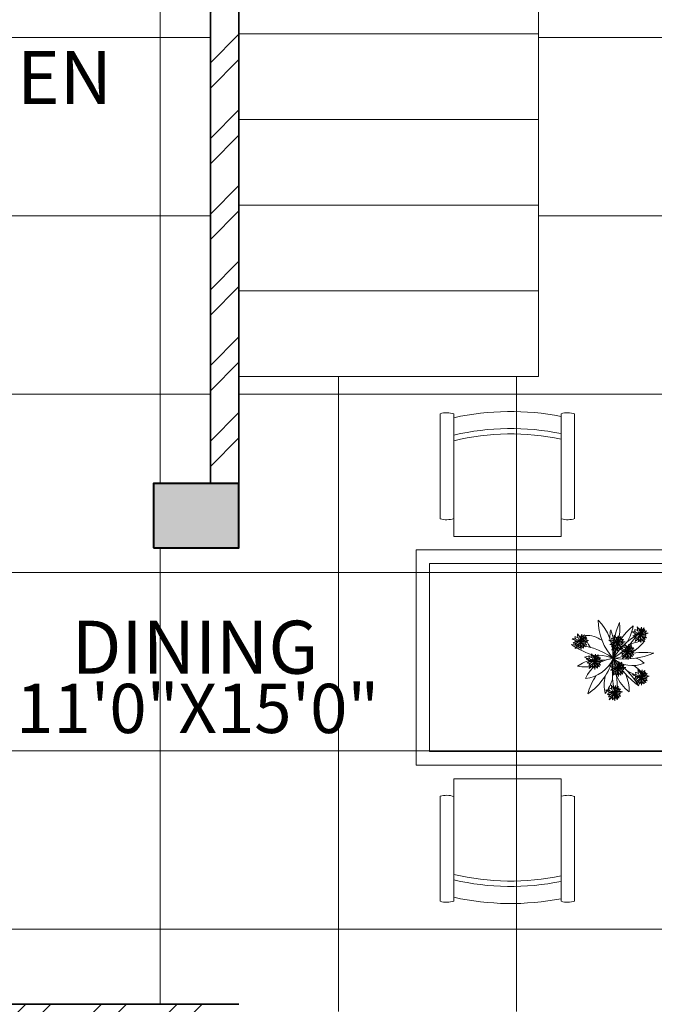
# Model space of a CAD drawing. Units: inches. Extents: x 351 to 1738, y -265 to 286.
# Tile 3 of 38: x 565 to 654, y 0 to 138. Entities that reach past the tile are written whole.
import ezdxf

# ---------------------------------------------------------------- set-up
doc = ezdxf.new("R2010")
doc.units = ezdxf.units.IN
doc.header["$MEASUREMENT"] = 0
for name, color, linetype, lineweight in [('A-AREA-IDEN', 7, 'Continuous', 18), ('A-COLS', 7, 'Continuous', 40), ('A-COLS-PATT', 6, 'Continuous', 13), ('A-FLOR-PATT', 9, 'Continuous', 9), ('A-FLOR-STRS', 7, 'Continuous', 18), ('A-FURN', 18, 'Continuous', 13), ('A-WALL', 7, 'Continuous', 35), ('A-WALL-PATT', 152, 'Continuous', 13)]:
    doc.layers.add(name, color=color, linetype=linetype, lineweight=lineweight)
doc.styles.add('Annotative', font='arial.ttf')

# ---------------------------------------------------------------- blocks, each defined once
blk = doc.blocks.new('CHAIR-DINING')
for p, q in [((0, 2.47), (0, 17.19)), ((18.84, 17.16), (18.84, 2.49))]:
    blk.add_line(p, q)
blk.add_lwpolyline([(16.96, 17.18), (16.96, 0), (1.88, 0), (1.88, 17.15)])
for centre, radius, start, end in [((0.89, 14.39), 2.93, 70.2624, 107.7226), ((9.88, -19.57), 37.07, 78.9982, 102.4562), ((17.86, 14.39), 2.93, 70.4535, 107.9116), ((9.88, -20.08), 35.19, 78.4012, 103.1346), ((9.88, -20.08), 34.43, 78.1438, 103.4274), ((0.89, 5.26), 2.93, 252.2774, 289.7376), ((17.89, 5.26), 2.93, 252.2774, 289.7376)]:
    blk.add_arc(centre, radius, start, end)
blk = doc.blocks.new('COL-9x12')
blk.add_lwpolyline([(0, 12), (0, 0), (9, 0), (9, 12)], close=True)

msp = doc.modelspace()

# ---------------------------------------------------------------- hatches: boundary and pattern name
at = {"layer": 'A-COLS-PATT'}
h = msp.add_hatch(color=256, dxfattribs=at)
h.dxf.hatch_style = 1
h.paths.add_polyline_path([(460.155, 237.963), (451.155, 237.963), (451.155, 228.963), (460.155, 228.963)])
h.paths.add_polyline_path([(463.155, 237.963), (460.155, 237.963), (460.155, 228.963), (463.155, 228.963)])
h.paths.add_polyline_path([(391.155, 255.963), (382.155, 255.963), (382.155, 243.963), (391.155, 243.963)])
h.paths.add_polyline_path([(391.155, 210.963), (382.155, 210.963), (382.155, 198.963), (391.155, 198.963)])
h.paths.add_polyline_path([(391.155, -45.037), (382.155, -45.037), (382.155, -57.037), (391.155, -57.037)])
h.paths.add_polyline_path([(460.155, -45.037), (451.155, -45.037), (451.155, -57.037), (460.155, -57.037)])
h.paths.add_polyline_path([(460.155, -161.037), (451.155, -161.037), (451.155, -164.037), (451.155, -173.037), (460.155, -173.037)])
h.paths.add_polyline_path([(391.155, -161.037), (382.155, -161.037), (382.155, -173.037), (391.155, -173.037)])
h.paths.add_polyline_path([(596, -164.037), (584, -164.037), (584, -173.037), (596, -173.037)])
h.paths.add_polyline_path([(596, -50), (584, -50), (584, -59), (596, -59)])
h.paths.add_polyline_path([(596.155, 73.463), (592.155, 73.463), (592.155, 64.463), (596.155, 64.463)])
h.paths.add_polyline_path([(592.155, 73.463), (584.155, 73.463), (584.155, 64.463), (592.155, 64.463)])
h.paths.add_polyline_path([(596.155, 237.963), (584.155, 237.963), (584.155, 228.963), (596.155, 228.963)])
h.paths.add_polyline_path([(739.655, 237.963), (727.655, 237.963), (727.655, 228.963), (739.655, 228.963)])
h.paths.add_polyline_path([(883.515, 237.963), (871.515, 237.963), (871.515, 228.963), (883.515, 228.963)])
h.paths.add_polyline_path([(883.515, 73.463), (871.515, 73.463), (871.515, 64.463), (883.515, 64.463)])
h.paths.add_polyline_path([(731.655, 73.463), (727.655, 73.463), (727.655, 64.463), (731.655, 64.463)])
h.paths.add_polyline_path([(739.515, 73.463), (731.655, 73.463), (731.655, 64.463), (739.515, 64.463)])
h.paths.add_polyline_path([(883.515, -53.037), (871.515, -53.037), (871.515, -57.037), (883.515, -57.037)])
h.paths.add_polyline_path([(883.515, -48.037), (871.515, -48.037), (871.515, -53.037), (883.515, -53.037)])
h.paths.add_polyline_path([(739.515, -48.037), (727.515, -48.037), (727.515, -56.5), (727.516, -57.037), (739.515, -57.037)])
h.paths.add_polyline_path([(883.515, -164.037), (871.515, -164.037), (871.515, -173.037), (883.515, -173.037)])
at = {"layer": 'A-FLOR-PATT', "transparency": 33554559}
h = msp.add_hatch(dxfattribs=at)
h.set_pattern_fill('ANSI37', color=256, scale=200, angle=45)
h.set_pattern_definition([(90, (460.077, -164.037), (-25, 0), []), (180, (460.077, -164.037), (-4e-15, -25), [])])
h.paths.add_polyline_path([(727.516, -57.037), (727.515, -57.037), (727.515, -56.5), (727.5, -45), (727.5, -3.5), (727.501, -2.537), (725.797, -2.537), (725.797, -3.037), (721.988, -3.037), (721.988, -2.537), (717.916, -2.537), (717.916, -3.037), (714.106, -3.037), (714.106, -2.537), (710.487, -2.537), (710.487, -3.037), (706.677, -3.037), (706.677, -2.537), (702.965, -2.537), (702.965, -3.037), (699.155, -3.037), (699.155, -2.537), (694.965, -2.537), (694.965, -3.037), (691.155, -3.037), (691.155, -2.537), (679.655, -2.537), (678.797, -2.537), (677.776, -2.537), (676.723, -2.537), (652.655, -2.537), (651.799, -2.537), (650.778, -2.537), (649.725, -2.537), (625.877, -2.537), (624.879, -2.537), (623.857, -2.537), (622.804, -2.537), (596.155, -2.537), (596.155, -3.537), (460.155, -3.537), (460.155, -81.037), (460.077, -99.07), (460.077, -133.967), (460.155, -152.037), (460.155, -164.037), (485.277, -164.037), (545.277, -164.037), (727.655, -164.037)])
h.paths.add_polyline_path([(584, -59), (584, -50), (596, -50), (596, -59)], flags=16)
h.paths.add_polyline_path([(905.155, 204.963), (731.655, 204.963), (731.655, 73.463), (739.515, 73.463), (739.515, 64.463), (731.655, 64.463), (731.655, -3.5), (727.655, -3.5), (727.655, -3.537), (727.5, -45), (731.655, -45), (731.655, -48.037), (739.515, -48.037), (739.515, -53.037), (754, -53.037), (754, -57.037), (748.655, -57.037), (748.655, -147.037), (815.655, -147.037), (815.655, -138.5), (819.655, -138.5), (819.655, -102.5), (815.655, -102.5), (815.655, -57.037), (790, -57.037), (790, -53.037), (871.515, -53.037), (871.515, -48.037), (883.515, -48.037), (883.515, -53.037), (905.155, -53.037)])
h.paths.add_polyline_path([(871.515, 64.463), (871.515, 73.463), (883.515, 73.463), (883.515, 64.463)], flags=16)
h.paths.add_polyline_path([(727.655, 64.463), (685.515, 64.463), (685.515, 186.963), (638.155, 186.963), (638.155, 88.463), (596.155, 88.463), (596.155, 64.463), (584.155, 64.463), (584.155, 73.463), (592.155, 73.463), (592.155, 205.963), (574, 205.963), (574, 209.963), (538, 209.963), (538, 205.963), (536.5, 205.963), (536.5, 180), (489.5, 180), (489.5, 68.655), (460.155, 68.655), (460.155, 64.463), (536.155, 64.463), (536.155, 48.463), (532.155, 48.463), (532.155, 60.463), (460.155, 60.463), (460.155, 0.463), (532.155, 0.463), (532.155, 12.463), (536.155, 12.463), (536.155, 0.463), (596.155, 0.463), (596.155, -0.537), (622.655, -0.537), (623.655, -0.537), (624.655, -0.537), (625.655, -0.537), (649.655, -0.537), (650.576, -0.537), (651.576, -0.537), (652.576, -0.537), (676.655, -0.537), (677.574, -0.537), (678.574, -0.537), (679.574, -0.537), (691.155, -0.537), (691.155, -0.037), (694.965, -0.037), (694.965, -0.537), (699.155, -0.537), (699.155, -0.037), (702.965, -0.037), (702.965, -0.537), (706.677, -0.537), (706.677, -0.037), (710.487, -0.037), (710.487, -0.537), (714.106, -0.537), (714.106, -0.037), (717.916, -0.037), (717.916, -0.537), (721.988, -0.537), (721.988, -0.037), (725.797, -0.037), (725.797, -0.537), (727.655, -0.537)])
h.paths.add_polyline_path([(485.401, 6.538), (461.783, 6.538), (461.783, 51.327), (485.401, 51.327)], flags=16)
h.paths.add_polyline_path([(483.401, 8.538), (463.783, 8.538), (463.783, 49.327), (483.401, 49.327)], flags=0)
h.paths.add_polyline_path([(476.907, 30.5), (476.907, 29.5), (476.907, 26), (475.907, 26), (475.907, 29.5), (474.449, 29.5), (474.449, 26), (473.449, 26), (470.5, 26), (470.5, 27), (473.449, 27), (473.449, 29.5), (470.5, 29.5), (470.5, 32.758), (471.5, 32.758), (471.5, 30.5), (473.407, 30.5), (473.407, 32.897), (473.407, 33.897), (476.907, 33.897), (476.907, 32.897), (474.407, 32.897), (474.407, 30.5)], flags=0)
at = {"layer": 'A-WALL-PATT'}
h = msp.add_hatch(dxfattribs=at)
h.set_pattern_fill('ANSI32', color=256, scale=20)
h.set_pattern_definition([(45, (382.155, -173.037), (-5.3033, 5.3033), []), (45, (385.691, -173.037), (-5.3033, 5.3033), [])])
h.paths.add_polyline_path([(391.155, -57.037), (382.155, -57.037), (382.155, -81.037), (391.155, -81.037)])
h.paths.add_polyline_path([(391.155, 198.963), (382.155, 198.963), (382.155, -45.037), (391.155, -45.037)])
h.paths.add_polyline_path([(391.155, 243.963), (382.155, 243.963), (382.155, 237.963), (382.155, 210.963), (391.155, 210.963)])
h.paths.add_polyline_path([(460.155, 255.963), (391.155, 255.963), (391.155, 246.963), (451.155, 246.963), (451.155, 237.963), (460.155, 237.963), (460.155, 251.963)])
h.paths.add_polyline_path([(404.155, 207.963), (391.155, 207.963), (391.155, 198.963), (404.155, 198.963)])
h.paths.add_polyline_path([(451.155, 207.963), (440.155, 207.963), (440.155, 198.963), (451.155, 198.963)])
h.paths.add_polyline_path([(460.155, 228.963), (451.155, 228.963), (451.155, 74.963), (460.155, 74.963), (460.155, 97.5)])
h.paths.add_polyline_path([(460.155, 60.463), (532.155, 60.463), (532.155, 48.463), (536.155, 48.463), (536.155, 64.463), (460.155, 64.463), (460.155, 62.963), (451.155, 62.963), (451.155, 46.258), (460.155, 46.258)])
h.paths.add_polyline_path([(460.155, -3.537), (596.155, -3.537), (596.155, 0.463), (536.155, 0.463), (536.155, 12.463), (532.155, 12.463), (532.155, 0.463), (460.155, 0.463), (460.155, 10.258), (451.155, 10.258), (451.155, -45.037), (460.155, -45.037)])
h.paths.add_polyline_path([(460.155, -57.037), (451.155, -57.037), (451.155, -81.037), (460.155, -81.037)])
h.paths.add_polyline_path([(460.155, -152.037), (451.155, -152.037), (451.155, -161.037), (460.155, -161.037)])
h.paths.add_polyline_path([(485.277, -164.037), (460.155, -164.037), (460.155, -164.5), (460.155, -173.037), (485.277, -173.037)])
h.paths.add_polyline_path([(584, -164.037), (545.277, -164.037), (545.277, -173.037), (584, -173.037)])
h.paths.add_polyline_path([(631.58, -164.037), (596, -164.037), (596, -173.037), (631.58, -173.037)])
h.paths.add_polyline_path([(871.515, -164.037), (819.655, -164.037), (819.655, -138.5), (815.655, -138.5), (815.655, -164.037), (691.58, -164.037), (691.58, -173.037), (871.515, -173.037)])
h.paths.add_polyline_path([(731.655, -57.037), (727.516, -57.037), (727.655, -164.037), (731.655, -164.037)])
h.paths.add_polyline_path([(914.155, -138), (905.155, -138), (905.155, -164.037), (883.515, -164.037), (883.515, -173.037), (914.155, -173.037)])
h.paths.add_polyline_path([(914.155, -30.189), (905.155, -30.189), (905.155, -53.037), (883.515, -53.037), (883.515, -57.037), (905.155, -57.037), (905.155, -102), (914.155, -102)])
h.paths.add_polyline_path([(871.515, -53.037), (790, -53.037), (790, -57.037), (815.655, -57.037), (815.655, -102.5), (819.655, -102.5), (819.655, -57.037), (871.515, -57.037)])
h.paths.add_polyline_path([(914.155, 120.993), (905.155, 120.993), (905.155, 29.811), (914.155, 29.811)])
h.paths.add_polyline_path([(731.655, 64.463), (727.655, 64.463), (727.655, -3.5), (731.655, -3.5)])
h.paths.add_polyline_path([(481.5, 209.963), (460.155, 209.963), (460.155, 205.963), (481.5, 205.963)])
h.paths.add_polyline_path([(538, 209.963), (517.5, 209.963), (517.5, 205.963), (538, 205.963)])
h.paths.add_polyline_path([(592.155, 209.963), (574, 209.963), (574, 205.963), (592.155, 205.963)])
h.paths.add_polyline_path([(596.155, 228.963), (592.155, 228.963), (592.155, 73.463), (596.155, 73.463)])
h.paths.add_polyline_path([(614, 237.963), (596.155, 237.963), (596.155, 228.963), (614, 228.963)])
h.paths.add_polyline_path([(677, 237.963), (650, 237.963), (650, 228.963), (677, 228.963)])
h.paths.add_polyline_path([(727.655, 237.963), (713, 237.963), (713, 228.963), (727.655, 228.963)])
h.paths.add_polyline_path([(871.515, 237.963), (739.655, 237.963), (739.655, 228.963), (871.515, 228.963)])
h.paths.add_polyline_path([(731.655, 228.963), (727.655, 228.963), (727.655, 73.463), (731.655, 73.463)])
h.paths.add_polyline_path([(914.155, 237.963), (883.515, 237.963), (883.515, 228.963), (905.155, 228.963), (905.155, 180.993), (914.155, 180.993)])

# ---------------------------------------------------------------- linework, layer by layer
at = {"layer": 'A-FLOR-STRS'}
for p, q in [((638.155, 88.463), (638.155, 228.963)), ((638.155, 136.463), (596.155, 136.463)), ((638.155, 124.463), (596.155, 124.463)), ((638.155, 112.463), (596.155, 112.463)), ((638.155, 100.463), (596.155, 100.463)), ((638.155, 88.463), (596.155, 88.463))]:
    msp.add_line(p, q, dxfattribs=at)
at = {"layer": 'A-FURN'}
for points in [[(677.515, 34), (677.515, 64.141), (621, 64.141), (621, 34)], [(675.631, 35.884), (675.631, 62.258), (622.884, 62.258), (622.884, 35.884)]]:
    msp.add_lwpolyline(points, close=True, dxfattribs=at)
for centre, radius, start, end in [((654.165, 54.2), 7.623, 179.15645, 223.43764), ((641.008, 49.071), 7.623, 359.15645, 43.43764), ((658.71, 49.745), 10.112, 155.37322, 184.46089), ((639.438, 53.172), 10.112, 335.37322, 4.46089), ((655.203, 51.553), 7.067, 168.46215, 178.29807), ((641.706, 50.372), 7.067, 348.46215, 21.54354), ((656.107, 47.477), 7.623, 127.80839, 168.79464), ((643.957, 54.981), 7.623, 330.60732, 348.79464), ((651.203, 50.618), 2.083, 54.66649, 88.96531), ((652.446, 54.401), 2.083, 234.66649, 253.95593), ((651.665, 52.206), 0.752, 55.6133, 92.65368), ((652.373, 53.069), 0.752, 188.55208, 216.30235), ((653.515, 53.366), 1.525, 179.15645, 223.43764), ((650.884, 52.34), 1.525, 359.15645, 43.43764), ((653.723, 52.837), 1.413, 168.46215, 178.29807), ((651.023, 52.601), 1.413, 348.46215, 21.54354), ((654.424, 52.475), 2.022, 155.37322, 184.46089), ((650.57, 53.161), 2.022, 335.37322, 4.46089), ((653.904, 52.022), 1.525, 127.80839, 168.79464), ((654.16, 51.204), 2.076, 121.28949, 147.55206), ((651.33, 54.092), 2.076, 301.28949, 327.55206), ((652.313, 53.531), 1.217, 274.47628, 323.76342), ((652.708, 54.54), 2.242, 262.30088, 292.02555), ((651.473, 53.522), 1.525, 330.60732, 348.79464), ((653.39, 51.598), 1.217, 94.47628, 115.35573), ((653.249, 50.239), 2.242, 82.30088, 99.71393), ((644.07, 53.403), 2.083, 234.66649, 253.95593), ((642.828, 49.62), 2.083, 54.66649, 88.96531), ((643.81, 49.955), 1.383, 105.54423, 124.46172), ((643.25, 52.46), 1.383, 260.74151, 281.17469), ((643.587, 50.186), 1.218, 68.55607, 107.25424), ((643.671, 52.483), 1.218, 248.55607, 287.25424), ((643.289, 51.208), 0.752, 55.6133, 92.65368), ((643.998, 52.071), 0.752, 188.55208, 216.30235), ((644.131, 50.366), 0.959, 95.89601, 156.10193), ((643.156, 51.708), 0.959, 275.89601, 336.10193), ((642.315, 51.796), 1.782, 304.27375, 344.50973), ((645.14, 52.368), 1.525, 179.15645, 223.43764), ((642.508, 51.342), 1.525, 359.15645, 43.43764), ((645.347, 51.839), 1.413, 168.46215, 178.29807), ((642.648, 51.603), 1.413, 348.46215, 21.54354), ((646.783, 50.96), 2.774, 172.53744, 196.15306), ((646.049, 51.477), 2.022, 155.37322, 184.46089), ((642.194, 52.163), 2.022, 335.37322, 4.46089), ((645.528, 51.024), 1.525, 127.80839, 168.79464), ((645.785, 50.206), 2.076, 121.28949, 147.55206), ((642.954, 53.094), 2.076, 301.28949, 327.55206), ((643.938, 52.533), 1.217, 274.47628, 323.76342), ((644.333, 53.542), 2.242, 262.30088, 292.02555), ((646.404, 52.807), 2.799, 212.08972, 233.74375), ((642.377, 49.063), 2.799, 32.08972, 53.74375), ((644.567, 51.914), 0.799, 228.05466, 294.46723), ((641.368, 50.548), 2.774, 352.53744, 16.15306), ((643.098, 52.524), 1.525, 330.60732, 348.79464), ((645.014, 50.6), 1.217, 94.47628, 115.35573), ((644.874, 49.241), 2.242, 82.30088, 99.71393), ((643.936, 50.124), 1.2, 34.96634, 55.81456), ((644.363, 50.593), 0.799, 48.05466, 66.71607), ((644.912, 48.399), 3.759, 55.6133, 92.65368), ((648.455, 52.714), 3.759, 188.55208, 216.30235), ((649.206, 53.203), 2.083, 234.66649, 253.95593), ((647.963, 49.421), 2.083, 54.66649, 88.96531), ((648.945, 49.755), 1.383, 105.54423, 124.46172), ((648.723, 49.986), 1.218, 68.55607, 107.25424), ((648.807, 52.284), 1.218, 248.55607, 287.25424), ((649.133, 51.871), 0.752, 188.55208, 216.30235), ((648.424, 51.008), 0.752, 55.6133, 92.65368), ((649.266, 50.166), 0.959, 95.89601, 156.10193), ((648.291, 51.509), 0.959, 275.89601, 336.10193), ((647.45, 51.596), 1.782, 304.27375, 344.50973), ((643.238, 57.83), 10.382, 301.28949, 327.55206), ((657.39, 43.388), 10.382, 121.28949, 147.55206), ((648.155, 55.026), 6.086, 274.47628, 323.76342), ((650.275, 52.169), 1.525, 179.15645, 223.43764), ((647.644, 51.143), 1.525, 359.15645, 43.43764), ((650.483, 51.639), 1.413, 168.46215, 178.29807), ((647.783, 51.403), 1.413, 348.46215, 21.54354), ((651.918, 50.76), 2.774, 172.53744, 196.15306), ((651.184, 51.278), 2.022, 155.37322, 184.46089), ((647.33, 51.963), 2.022, 335.37322, 4.46089), ((650.663, 50.824), 1.525, 127.80839, 168.79464), ((650.92, 50.006), 2.076, 121.28949, 147.55206), ((648.09, 52.895), 2.076, 301.28949, 327.55206), ((649.073, 52.334), 1.217, 274.47628, 323.76342), ((649.468, 53.342), 2.242, 262.30088, 292.02555), ((651.539, 52.607), 2.799, 212.08972, 233.74375), ((647.513, 48.863), 2.799, 32.08972, 53.74375), ((649.702, 51.714), 0.799, 228.05466, 294.46723), ((646.504, 50.349), 2.774, 352.53744, 16.15306), ((648.233, 52.325), 1.525, 330.60732, 348.79464), ((650.15, 50.401), 1.217, 94.47628, 115.35573), ((650.009, 49.042), 2.242, 82.30088, 99.71393), ((649.499, 50.393), 0.799, 48.05466, 66.71607), ((653.538, 45.361), 6.086, 94.47628, 115.35573), ((652.186, 50.953), 1.383, 105.54423, 124.46172), ((651.625, 53.458), 1.383, 260.74151, 281.17469), ((651.963, 51.184), 1.218, 68.55607, 107.25424), ((652.047, 53.481), 1.218, 248.55607, 287.25424), ((652.507, 51.364), 0.959, 95.89601, 156.10193), ((651.531, 52.706), 0.959, 275.89601, 336.10193), ((650.69, 52.794), 1.782, 304.27375, 344.50973), ((653.412, 50.845), 1.782, 146.31237, 164.50973), ((653.373, 51.576), 1.217, 168.71287, 191.75798), ((651.216, 52.07), 1.217, 322.47084, 344.98088), ((655.158, 51.958), 2.774, 172.53744, 196.15306), ((652.942, 52.912), 0.799, 228.05466, 294.46723), ((654.779, 53.805), 2.799, 212.08972, 233.74375), ((650.753, 50.061), 2.799, 32.08972, 53.74375), ((649.744, 51.546), 2.774, 352.53744, 16.15306), ((653.56, 52.29), 1.153, 203.44868, 232.2657), ((651.703, 51.406), 1.153, 358.59558, 23.61242), ((653.392, 53.006), 1.2, 241.30744, 265.38561), ((652.312, 51.122), 1.2, 34.96634, 55.81456), ((652.739, 51.591), 0.799, 48.05466, 66.71607), ((642.605, 40.461), 10.416, 54.66649, 88.96531), ((648.818, 59.373), 10.416, 234.66649, 253.95593), ((645.036, 49.847), 1.782, 146.31237, 164.50973), ((644.998, 50.578), 1.217, 168.71287, 191.75798), ((642.841, 51.072), 1.217, 322.47084, 344.98088), ((645.185, 51.292), 1.153, 203.44868, 232.2657), ((643.327, 50.408), 1.153, 358.59558, 23.61242), ((645.016, 52.008), 1.2, 241.30744, 265.38561), ((648.385, 52.261), 1.383, 260.74151, 281.17469), ((650.172, 49.647), 1.782, 146.31237, 164.50973), ((650.133, 50.379), 1.217, 168.71287, 191.75798), ((647.976, 50.872), 1.217, 322.47084, 344.98088), ((650.32, 51.092), 1.153, 203.44868, 232.2657), ((650.668, 52.006), 2.083, 234.66649, 253.95593), ((649.426, 48.223), 2.083, 54.66649, 88.96531), ((648.462, 50.209), 1.153, 358.59558, 23.61242), ((650.151, 51.808), 1.2, 241.30744, 265.38561), ((650.408, 48.558), 1.383, 105.54423, 124.46172), ((649.848, 51.063), 1.383, 260.74151, 281.17469), ((649.071, 49.924), 1.2, 34.96634, 55.81456), ((650.185, 48.789), 1.218, 68.55607, 107.25424), ((650.269, 51.086), 1.218, 248.55607, 287.25424), ((649.887, 49.811), 0.752, 55.6133, 92.65368), ((650.596, 50.674), 0.752, 188.55208, 216.30235), ((650.729, 48.969), 0.959, 95.89601, 156.10193), ((649.754, 50.311), 0.959, 275.89601, 336.10193), ((648.913, 50.399), 1.782, 304.27375, 344.50973), ((651.738, 50.971), 1.525, 179.15645, 223.43764), ((649.106, 49.945), 1.525, 359.15645, 43.43764), ((651.945, 50.442), 1.413, 168.46215, 178.29807), ((649.246, 50.205), 1.413, 348.46215, 21.54354), ((653.381, 49.562), 2.774, 172.53744, 196.15306), ((652.647, 50.08), 2.022, 155.37322, 184.46089), ((648.792, 50.765), 2.022, 335.37322, 4.46089), ((652.126, 49.626), 1.525, 127.80839, 168.79464), ((652.383, 48.809), 2.076, 121.28949, 147.55206), ((649.552, 51.697), 2.076, 301.28949, 327.55206), ((650.536, 51.136), 1.217, 274.47628, 323.76342), ((650.931, 52.145), 2.242, 262.30088, 292.02555), ((653.002, 51.41), 2.799, 212.08972, 233.74375), ((648.975, 47.666), 2.799, 32.08972, 53.74375), ((647.967, 49.151), 2.774, 352.53744, 16.15306), ((651.165, 50.517), 0.799, 228.05466, 294.46723), ((652.834, 38.565), 11.212, 82.30088, 99.71393), ((649.696, 51.127), 1.525, 330.60732, 348.79464), ((651.612, 49.203), 1.217, 94.47628, 115.35573), ((651.472, 47.844), 2.242, 82.30088, 99.71393), ((650.534, 48.726), 1.2, 34.96634, 55.81456), ((650.962, 49.196), 0.799, 48.05466, 66.71607), ((647.517, 42.133), 6.916, 105.54423, 124.46172), ((646.402, 43.289), 6.092, 68.55607, 107.25424), ((646.823, 54.776), 6.092, 248.55607, 287.25424), ((649.122, 44.189), 4.795, 95.89601, 156.10193), ((644.245, 50.901), 4.795, 275.89601, 336.10193), ((646.02, 50.608), 2.083, 234.66649, 253.95593), ((644.778, 46.826), 2.083, 54.66649, 88.96531), ((645.76, 47.16), 1.383, 105.54423, 124.46172), ((645.2, 49.666), 1.383, 260.74151, 281.17469), ((640.041, 51.339), 8.912, 304.27375, 344.50973), ((645.537, 47.391), 1.218, 68.55607, 107.25424), ((645.621, 49.689), 1.218, 248.55607, 287.25424), ((645.239, 48.414), 0.752, 55.6133, 92.65368), ((645.948, 49.277), 0.752, 188.55208, 216.30235), ((646.081, 47.572), 0.959, 95.89601, 156.10193), ((645.106, 48.914), 0.959, 275.89601, 336.10193), ((644.265, 49.002), 1.782, 304.27375, 344.50973), ((644.458, 48.548), 1.525, 359.15645, 43.43764), ((647.09, 49.574), 1.525, 179.15645, 223.43764), ((647.297, 49.044), 1.413, 168.46215, 178.29807), ((644.598, 48.808), 1.413, 348.46215, 21.54354), ((648.733, 48.165), 2.774, 172.53744, 196.15306), ((647.999, 48.683), 2.022, 155.37322, 184.46089), ((644.144, 49.368), 2.022, 335.37322, 4.46089), ((647.478, 48.229), 1.525, 127.80839, 168.79464), ((647.735, 47.411), 2.076, 121.28949, 147.55206), ((644.904, 50.3), 2.076, 301.28949, 327.55206), ((645.888, 49.739), 1.217, 274.47628, 323.76342), ((646.283, 50.748), 2.242, 262.30088, 292.02555), ((643.318, 47.754), 2.774, 352.53744, 16.15306), ((648.354, 50.012), 2.799, 212.08972, 233.74375), ((644.327, 46.268), 2.799, 32.08972, 53.74375), ((646.517, 49.12), 0.799, 228.05466, 294.46723), ((645.048, 49.73), 1.525, 330.60732, 348.79464), ((646.964, 47.806), 1.217, 94.47628, 115.35573), ((646.824, 46.447), 2.242, 82.30088, 99.71393), ((645.886, 47.329), 1.2, 34.96634, 55.81456), ((646.314, 47.798), 0.799, 48.05466, 66.71607), ((662.381, 47.157), 13.869, 172.53744, 196.15306), ((650.132, 60.069), 11.212, 262.30088, 292.02555), ((640.353, 37.673), 13.995, 32.08972, 53.74375), ((635.308, 45.1), 13.869, 352.53744, 16.15306), ((651.299, 51.929), 3.994, 228.05466, 294.46723), ((660.486, 56.393), 13.995, 212.08972, 233.74375), ((650.37, 48.576), 1.525, 179.15645, 223.43764), ((647.739, 47.55), 1.525, 359.15645, 43.43764), ((650.578, 48.046), 1.413, 168.46215, 178.29807), ((647.878, 47.81), 1.413, 348.46215, 21.54354), ((651.279, 47.685), 2.022, 155.37322, 184.46089), ((647.425, 48.37), 2.022, 335.37322, 4.46089), ((650.758, 47.231), 1.525, 127.80839, 168.79464), ((648.328, 48.732), 1.525, 330.60732, 348.79464), ((651.635, 48.45), 1.782, 146.31237, 164.50973), ((651.596, 49.181), 1.217, 168.71287, 191.75798), ((649.439, 49.675), 1.217, 322.47084, 344.98088), ((651.783, 49.894), 1.153, 203.44868, 232.2657), ((649.925, 49.011), 1.153, 358.59558, 23.61242), ((651.614, 50.611), 1.2, 241.30744, 265.38561), ((650.284, 45.323), 3.994, 48.05466, 66.71607), ((644.716, 54.66), 6.916, 260.74151, 281.17469), ((646.986, 47.053), 1.782, 146.31237, 164.50973), ((646.948, 47.784), 1.217, 168.71287, 191.75798), ((644.791, 48.277), 1.217, 322.47084, 344.98088), ((647.135, 48.497), 1.153, 203.44868, 232.2657), ((645.277, 47.614), 1.153, 358.59558, 23.61242), ((646.966, 49.213), 1.2, 241.30744, 265.38561), ((648.058, 45.828), 2.083, 54.66649, 88.96531), ((649.301, 49.61), 2.083, 234.66649, 253.95593), ((649.04, 46.162), 1.383, 105.54423, 124.46172), ((648.48, 48.668), 1.383, 260.74151, 281.17469), ((648.818, 46.393), 1.218, 68.55607, 107.25424), ((648.902, 48.691), 1.218, 248.55607, 287.25424), ((648.519, 47.416), 0.752, 55.6133, 92.65368), ((649.228, 48.279), 0.752, 188.55208, 216.30235), ((649.361, 46.574), 0.959, 95.89601, 156.10193), ((648.386, 47.916), 0.959, 275.89601, 336.10193), ((647.545, 48.004), 1.782, 304.27375, 344.50973), ((650.267, 46.055), 1.782, 146.31237, 164.50973), ((650.228, 46.786), 1.217, 168.71287, 191.75798), ((648.071, 47.279), 1.217, 322.47084, 344.98088), ((652.013, 47.167), 2.774, 172.53744, 196.15306), ((651.015, 46.413), 2.076, 121.28949, 147.55206), ((648.185, 49.302), 2.076, 301.28949, 327.55206), ((649.168, 48.741), 1.217, 274.47628, 323.76342), ((649.563, 49.75), 2.242, 262.30088, 292.02555), ((649.797, 48.122), 0.799, 228.05466, 294.46723), ((647.608, 45.27), 2.799, 32.08972, 53.74375), ((651.634, 49.014), 2.799, 212.08972, 233.74375), ((646.599, 46.756), 2.774, 352.53744, 16.15306), ((650.415, 47.499), 1.153, 203.44868, 232.2657), ((648.557, 46.616), 1.153, 358.59558, 23.61242), ((650.246, 48.215), 1.2, 241.30744, 265.38561), ((650.245, 46.808), 1.217, 94.47628, 115.35573), ((650.104, 45.449), 2.242, 82.30088, 99.71393), ((649.166, 46.331), 1.2, 34.96634, 55.81456), ((649.594, 46.8), 0.799, 48.05466, 66.71607), ((653.547, 52.398), 6.001, 241.30744, 265.38561), ((648.147, 42.977), 6.001, 34.96634, 55.81456), ((651.768, 46.218), 0.752, 55.6133, 92.65368), ((652.476, 47.081), 0.752, 188.55208, 216.30235), ((653.618, 47.378), 1.525, 179.15645, 223.43764), ((650.987, 46.352), 1.525, 359.15645, 43.43764), ((653.826, 46.849), 1.413, 168.46215, 178.29807), ((651.126, 46.613), 1.413, 348.46215, 21.54354), ((654.527, 46.487), 2.022, 155.37322, 184.46089), ((650.673, 47.173), 2.022, 335.37322, 4.46089), ((654.007, 46.034), 1.525, 127.80839, 168.79464), ((654.263, 45.216), 2.076, 121.28949, 147.55206), ((651.433, 48.104), 2.076, 301.28949, 327.55206), ((651.577, 47.534), 1.525, 330.60732, 348.79464), ((653.648, 41.594), 8.912, 146.31237, 164.50973), ((653.456, 45.251), 6.086, 168.71287, 191.75798), ((642.671, 47.718), 6.086, 322.47084, 344.98088), ((654.392, 48.817), 5.764, 203.44868, 232.2657), ((645.102, 44.4), 5.764, 358.59558, 23.61242), ((651.306, 44.63), 2.083, 54.66649, 88.96531), ((652.549, 48.413), 2.083, 234.66649, 253.95593), ((652.289, 44.965), 1.383, 105.54423, 124.46172), ((651.728, 47.47), 1.383, 260.74151, 281.17469), ((652.066, 45.196), 1.218, 68.55607, 107.25424), ((652.15, 47.493), 1.218, 248.55607, 287.25424), ((652.61, 45.376), 0.959, 95.89601, 156.10193), ((651.634, 46.718), 0.959, 275.89601, 336.10193), ((650.793, 46.806), 1.782, 304.27375, 344.50973), ((653.515, 44.857), 1.782, 146.31237, 164.50973), ((653.476, 45.588), 1.217, 168.71287, 191.75798), ((651.32, 46.082), 1.217, 322.47084, 344.98088), ((655.261, 45.97), 2.774, 172.53744, 196.15306), ((652.416, 47.543), 1.217, 274.47628, 323.76342), ((652.812, 48.552), 2.242, 262.30088, 292.02555), ((653.045, 46.924), 0.799, 228.05466, 294.46723), ((654.882, 47.817), 2.799, 212.08972, 233.74375), ((650.856, 44.073), 2.799, 32.08972, 53.74375), ((649.847, 45.558), 2.774, 352.53744, 16.15306), ((653.664, 46.302), 1.153, 203.44868, 232.2657), ((651.806, 45.418), 1.153, 358.59558, 23.61242), ((653.495, 47.018), 1.2, 241.30744, 265.38561), ((653.493, 45.61), 1.217, 94.47628, 115.35573), ((653.352, 44.251), 2.242, 82.30088, 99.71393), ((652.415, 45.134), 1.2, 34.96634, 55.81456), ((652.842, 45.603), 0.799, 48.05466, 66.71607), ((647.564, 42.435), 2.083, 54.66649, 88.96531), ((648.807, 46.217), 2.083, 234.66649, 253.95593), ((648.324, 43), 1.218, 68.55607, 107.25424), ((648.408, 45.298), 1.218, 248.55607, 287.25424), ((648.026, 44.023), 0.752, 55.6133, 92.65368), ((648.734, 44.885), 0.752, 188.55208, 216.30235), ((649.876, 45.183), 1.525, 179.15645, 223.43764), ((647.245, 44.157), 1.525, 359.15645, 43.43764), ((650.084, 44.653), 1.413, 168.46215, 178.29807), ((647.384, 44.417), 1.413, 348.46215, 21.54354), ((650.785, 44.292), 2.022, 155.37322, 184.46089), ((646.931, 44.977), 2.022, 335.37322, 4.46089), ((650.265, 43.838), 1.525, 127.80839, 168.79464), ((647.691, 45.909), 2.076, 301.28949, 327.55206), ((650.521, 43.02), 2.076, 121.28949, 147.55206), ((648.674, 45.348), 1.217, 274.47628, 323.76342), ((649.069, 46.356), 2.242, 262.30088, 292.02555), ((647.835, 45.339), 1.525, 330.60732, 348.79464), ((649.751, 43.415), 1.217, 94.47628, 115.35573), ((649.61, 42.056), 2.242, 82.30088, 99.71393), ((648.547, 42.769), 1.383, 105.54423, 124.46172), ((647.986, 45.275), 1.383, 260.74151, 281.17469), ((648.868, 43.18), 0.959, 95.89601, 156.10193), ((647.892, 44.523), 0.959, 275.89601, 336.10193), ((647.051, 44.61), 1.782, 304.27375, 344.50973), ((649.773, 42.661), 1.782, 146.31237, 164.50973), ((649.734, 43.393), 1.217, 168.71287, 191.75798), ((647.577, 43.886), 1.217, 322.47084, 344.98088), ((651.519, 43.774), 2.774, 172.53744, 196.15306), ((647.114, 41.877), 2.799, 32.08972, 53.74375), ((651.14, 45.621), 2.799, 212.08972, 233.74375), ((646.105, 43.363), 2.774, 352.53744, 16.15306), ((649.303, 44.728), 0.799, 228.05466, 294.46723), ((649.921, 44.106), 1.153, 203.44868, 232.2657), ((648.064, 43.223), 1.153, 358.59558, 23.61242), ((649.753, 44.822), 1.2, 241.30744, 265.38561), ((648.673, 42.938), 1.2, 34.96634, 55.81456), ((649.1, 43.407), 0.799, 48.05466, 66.71607)]:
    msp.add_arc(centre, radius, start, end, dxfattribs=at)
at = {"layer": 'A-WALL'}
for p, q in [((596.155, 237.963), (596.155, 64.463)), ((592.155, 228.963), (592.155, 73.463)), ((592.155, 64.463), (596.155, 64.463)), ((536.155, 0.463), (596.155, 0.463))]:
    msp.add_line(p, q, dxfattribs=at)

# ---------------------------------------------------------------- block references
at = {"layer": 'A-COLS', "rotation": 90.00000000000082}
msp.add_blockref('COL-9x12', (596.155, 64.462), dxfattribs=at)
at = {"layer": 'A-FURN'}
msp.add_blockref('CHAIR-DINING', (624.383, 66.054), dxfattribs=at)
at = {"layer": 'A-FURN', "extrusion": (0, 0, -1), "zscale": -1, "rotation": 180}
msp.add_blockref('CHAIR-DINING', (-624.383, 32.087), dxfattribs=at)

# ---------------------------------------------------------------- texts
at = {"layer": 'A-AREA-IDEN', "style": 'Annotative'}
for s, height, p in [('OPEN KITCHEN', 7.43256, (506.097, 126.656)), ('DINING', 7.4326, (572.705, 46.798)), ('11\'0"X15\'0"', 6.90137, (564.919, 38.486))]:
    msp.add_text(s, height=height, dxfattribs=at).set_placement(p)

doc.saveas('drawing.dxf')
